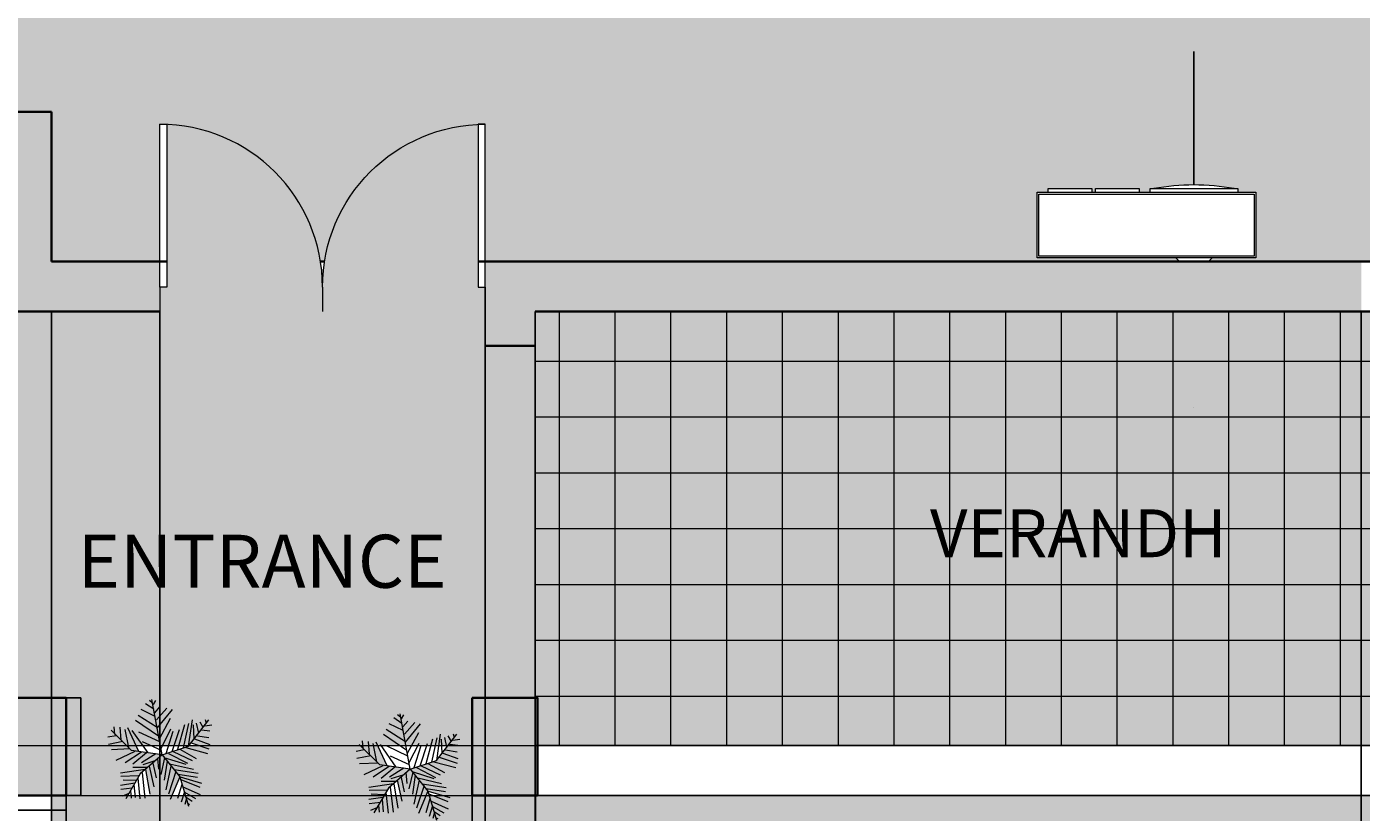
# Model space of a CAD drawing. Units: millimetres. Extents: x -229 to 16545, y -10488 to 4272.
# Tile 7 of 29: x 5862 to 12015, y -7746 to -4126. Entities that reach past the tile are written whole.
import ezdxf

# ---------------------------------------------------------------- set-up
doc = ezdxf.new("R2010")
doc.units = ezdxf.units.MM
for name, color, linetype, lineweight in [('A-ANNO-DIMS', 2, 'Continuous', 18), ('A-AREA-IDEN', 7, 'Continuous', 18), ('A-COLS', 7, 'Continuous', 35), ('A-DOOR', 4, 'Continuous', 18), ('A-FLOR-STRS', 7, 'Continuous', 18), ('A-FURN', 8, 'Continuous', 18), ('A-WALL', 7, 'Continuous', 35), ('L-PLNT-BEDS', 82, 'Continuous', 18), ('L-PLNT-TREE', 80, 'Continuous', 18), ('L-PVMT', 7, 'Continuous', 18), ('L-PVMT-JNTS', 8, 'Continuous', 13)]:
    doc.layers.add(name, color=color, linetype=linetype, lineweight=lineweight)
for name, color, linetype, lineweight, true_color in [('A-FLOR-PATT', 254, 'Continuous', 13, 0xfeeab9), ('A-FLOR-STRS-PATT', 51, 'Continuous', 13, 0xf8f6b0), ('A-WALL-PATT', 18, 'Continuous', 13, 0x000000), ('L-PLNT-PATT', 116, 'Continuous', 13, 0x136734), ('L-PVMT-PATT', 252, 'Continuous', 13, 0x939598)]:
    doc.layers.add(name, color=color, linetype=linetype, lineweight=lineweight, true_color=true_color)
doc.styles.get("Standard").update_dxf_attribs({"font": 'arial.ttf'})
doc.dimstyles.get("Standard").update_dxf_attribs({"dimtxt": 0.18, "dimasz": 0.18, "dimexe": 0.18, "dimexo": 0.0625, "dimgap": 0.09, "dimtad": 0, "dimtih": 1, "dimtoh": 1, "dimdec": 4, "dimzin": 0, "dimdsep": 46, "dimtxsty": 'Standard', "dimcen": 0.09, "dimadec": 0, "dimazin": 0, "dimtfac": 1, "dimtdec": 4, "dimtofl": 0, "dimtmove": 0, "dimatfit": 3, "dimfxl": 1, "dimtolj": 1, "dimtzin": 0, "dimarcsym": 0})

# ---------------------------------------------------------------- blocks, each defined once
blk = doc.blocks.new('Entertainment Center')
for p, q in [((-4, 0), (-5, -1)), ((4, 0), (-4, 0)), ((5, -1), (4, 0)), ((-17, -19), (-17, -1)), ((-17, -1), (43, -1)), ((-16.5, -18.5), (-16.5, -1.5)), ((-16.5, -1.5), (42.5, -1.5)), ((42.5, -1.5), (42.5, -18.5)), ((43, -1), (43, -19)), ((43, -19), (-17, -19)), ((42.5, -18.5), (-16.5, -18.5)), ((-12, -20), (-12, -19)), ((12, -20), (-12, -20)), ((12, -19), (12, -20)), ((15, -20), (15, -19)), ((27, -20), (15, -20)), ((27, -19), (27, -20)), ((28, -20), (28, -19)), ((40, -20), (28, -20)), ((40, -19), (40, -20))]:
    blk.add_line(p, q)
blk.add_arc((0, 40), 61, 259.6111, 280.3889)
blk = doc.blocks.new('*U12')
for p, q in [((0, 0), (0, -6)), ((40, 0), (40, -6))]:
    blk.add_line(p, q)
blk.add_lwpolyline([(0, 0), (0, 40), (1.75, 40), (1.75, 0)], close=True)
blk.add_arc((0, 0), 40, 0, 90)
blk = doc.blocks.new('*U18')
for p, q in [((-10.186, 53.64), (-13.084, 55.962)), ((0, 0), (-10.5, 57)), ((-9.099, 51.782), (-6.563, 55.962)), ((-7.288, 39.707), (-21.778, 46.673)), ((-8.737, 47.138), (-17.069, 52.711)), ((-7.65, 43.423), (-2.578, 49.46)), ((-5.839, 35.992), (4.667, 48.067)), ((-5.114, 27.632), (10.463, 46.673)), ((-48.585, 21.131), (-49.309, 29.026)), ((-43.513, 28.561), (-42.427, 15.558)), ((-35.544, 28.097), (-24.314, 3.947)), ((-3.665, 19.273), (-27.574, 35.527)), ((-5.114, 28.097), (-24.676, 40.636)), ((-2.941, 16.486), (8.652, 37.85)), ((16.259, 5.805), (23.142, 31.348)), ((22.055, 7.198), (27.489, 32.277)), ((27, 9), (48, 36)), ((27.127, 9.056), (31.112, 35.992)), ((31.836, 30.883), (32.561, 16.486)), ((35.096, 32.741), (37.27, 22.524)), ((38.719, 34.134), (41.979, 28.561)), ((43.791, 29.954), (51.036, 30.883)), ((44.153, 36.456), (45.239, 32.741)), ((-47.498, 19.737), (-55.83, 18.344)), ((-31.5, 4.5), (-52.5, 25.5)), ((-38.442, 26.239), (-34.819, 7.663)), ((-14.533, 2.09), (-30.834, 25.31)), ((-24.314, 23.917), (-2.941, 13.7)), ((-1.129, 6.734), (9.014, 26.704)), ((3.942, 1.625), (11.187, 24.381)), ((10.101, 3.483), (17.708, 26.239)), ((33.285, 16.486), (48.862, 10.913)), ((36.183, 19.737), (48.137, 17.88)), ((40.53, 25.775), (48.862, 24.846)), ((-40.615, 13.7), (-55.105, 10.913)), ((-33.37, 6.269), (-52.207, 5.34)), ((-28.299, 3.483), (-47.86, -5.805)), ((-21.416, 3.018), (-38.079, -8.128)), ((0, 0), (-31.5, 4.5)), ((-15.982, 2.09), (-30.11, -9.521)), ((0, 0), (-22.5, -19.5)), ((-6.563, 1.161), (-21.416, -8.128)), ((-20.691, 13.7), (-1.129, 4.876)), ((0, 0), (27, 9)), ((0, 0), (18, -22.5)), ((6.478, 1.625), (26.04, -8.592)), ((11.187, 3.483), (30.749, -5.805)), ((18.07, 5.805), (35.096, -3.483)), ((24.229, 7.663), (46.688, 1.625)), ((29.662, 12.307), (48.137, 6.269)), ((-15.257, -12.772), (-30.11, -12.772)), ((-6.563, -5.805), (-19.967, -9.985)), ((-13.446, -11.378), (-8.737, -32.741)), ((-9.461, -8.592), (-6.201, -23.453)), ((-4.752, -3.483), (-3.665, -14.629)), ((2.493, -3.019), (-1.491, -20.202)), ((1.769, -2.555), (24.229, -9.521)), ((5.029, -6.27), (2.131, -25.775)), ((9.014, -11.378), (3.58, -35.992)), ((7.565, -9.056), (32.198, -14.629)), ((-17.431, -15.094), (-42.789, -18.809)), ((-24.314, -21.596), (-42.427, -22.06)), ((-26.849, -26.24), (-40.253, -25.775)), ((-22.5, -19.5), (-37.5, -45)), ((-25.038, -23.918), (-22.865, -45.281)), ((-20.691, -18.345), (-17.793, -44.352)), ((-17.069, -15.094), (-12.721, -40.172)), ((14.085, -16.951), (6.478, -40.172)), ((18.07, -22.524), (8.289, -45.745)), ((12.274, -15.094), (36.907, -18.809)), ((16.259, -19.738), (36.183, -22.989)), ((18, -22.5), (27, -52.5)), ((18.433, -22.524), (40.53, -29.026)), ((19.157, -25.311), (38.719, -33.206)), ((-28.299, -29.026), (-42.789, -31.348)), ((-30.834, -34.135), (-42.427, -35.528)), ((-34.457, -39.708), (-40.978, -42.494)), ((-32.646, -36.921), (-31.921, -44.352)), ((-29.023, -30.884), (-27.936, -43.887)), ((20.244, -30.419), (15.897, -44.816)), ((22.78, -37.85), (19.519, -48.532)), ((21.331, -32.741), (39.081, -40.636)), ((22.78, -38.314), (34.372, -44.816)), ((24.591, -45.745), (23.142, -50.854)), ((24.591, -43.423), (30.749, -47.603)), ((26.764, -49.925), (28.213, -50.854))]:
    blk.add_line(p, q)
blk = doc.blocks.new('COL-300x450')
at = {"transparency": 33554615}
h = blk.add_hatch(color=256, dxfattribs=at)
h.dxf.hatch_style = 1
h.paths.add_polyline_path([(300, 450), (0, 450), (0, 0), (300, 0)])
at = {"transparency": 33554687}
blk.add_lwpolyline([(0, 450), (300, 450), (300, 0), (0, 0)], close=True, dxfattribs=at)
blk = doc.blocks.new('*D23')
at = {"layer": 'A-ANNO-DIMS', "color": 0, "lineweight": -2, "transparency": 16777216}
for p, q in [((6043.9, -7218.3), (6111.5, -7218.3)), ((6111.4, -7218.5), (6111.4, -7443.1)), ((6111.4, -7668.1), (6111.4, -7443.5)), ((6043.9, -7668.3), (6111.5, -7668.3))]:
    blk.add_line(p, q, dxfattribs=at)
at = {"layer": 'A-ANNO-DIMS', "color": 0, "transparency": 16777216}
for points in [[(6111.3, -7218.5), (6111.4, -7218.5), (6111.4, -7218.3)], [(6111.3, -7668.1), (6111.4, -7668.1), (6111.4, -7668.3)]]:
    blk.add_solid(points, dxfattribs=at)
at = {"layer": 'Defpoints', "color": 0, "transparency": 16777216}
for p in [(6043.9, -7218.3), (6111.4, -7218.3), (6043.9, -7668.3)]:
    blk.add_point(p, dxfattribs=at)
at = {"layer": 'A-ANNO-DIMS', "color": 0, "transparency": 16777216, "insert": (6111.4, -7443.3), "char_height": 0.18, "attachment_point": 5}
blk.add_mtext('\\A1;COLUMN 450 TYP.', dxfattribs=at)
blk = doc.blocks.new('*D24')
at = {"layer": 'A-ANNO-DIMS', "color": 0, "lineweight": -2, "transparency": 16777216}
for p, q in [((5743.9, -7668.3), (5743.9, -7736)), ((6043.9, -7668.3), (6043.9, -7736)), ((5744, -7735.8), (5893.3, -7735.8)), ((6043.7, -7735.8), (5894.5, -7735.8))]:
    blk.add_line(p, q, dxfattribs=at)
at = {"layer": 'A-ANNO-DIMS', "color": 0, "transparency": 16777216}
for points in [[(5744, -7735.7), (5744, -7735.8), (5743.9, -7735.8)], [(6043.7, -7735.7), (6043.7, -7735.8), (6043.9, -7735.8)]]:
    blk.add_solid(points, dxfattribs=at)
at = {"layer": 'Defpoints', "color": 0, "transparency": 16777216}
for p in [(5743.9, -7668.3), (6043.9, -7668.3), (6043.9, -7735.8)]:
    blk.add_point(p, dxfattribs=at)
at = {"layer": 'A-ANNO-DIMS', "color": 0, "transparency": 16777216, "insert": (5893.9, -7735.8), "char_height": 0.18, "attachment_point": 5}
blk.add_mtext('\\A1;300 TYP.', dxfattribs=at)
blk = doc.blocks.new('*D60')
at = {"layer": 'A-ANNO-DIMS', "color": 0, "lineweight": -2, "transparency": 16777216}
for p, q in [((8205.9, -7438.3), (8205.9, -10230.2)), ((14015.9, -7438.3), (14015.9, -10230.2)), ((8206.1, -10230), (11110.6, -10230)), ((14015.8, -10230), (11111.3, -10230))]:
    blk.add_line(p, q, dxfattribs=at)
at = {"layer": 'A-ANNO-DIMS', "color": 0, "transparency": 16777216}
for points in [[(8206.1, -10230), (8206.1, -10230.1), (8205.9, -10230)], [(14015.8, -10230), (14015.8, -10230.1), (14015.9, -10230)]]:
    blk.add_solid(points, dxfattribs=at)
at = {"layer": 'Defpoints', "color": 0, "transparency": 16777216}
for p in [(8205.9, -7438.3), (14015.9, -7438.3), (14015.9, -10230)]:
    blk.add_point(p, dxfattribs=at)
at = {"layer": 'A-ANNO-DIMS', "color": 0, "transparency": 16777216, "insert": (11110.9, -10230), "char_height": 0.18, "attachment_point": 5}
blk.add_mtext('\\A1;5810', dxfattribs=at)
blk = doc.blocks.new('*D61')
at = {"layer": 'A-ANNO-DIMS', "color": 0, "lineweight": -2, "transparency": 16777216}
for p, q in [((8206, -5438.3), (16544.5, -5438.3)), ((16544.3, -5438.5), (16544.3, -6438.1)), ((16544.3, -7438.1), (16544.3, -6438.5)), ((8206, -7438.3), (16544.5, -7438.3))]:
    blk.add_line(p, q, dxfattribs=at)
at = {"layer": 'A-ANNO-DIMS', "color": 0, "transparency": 16777216}
for points in [[(16544.3, -5438.5), (16544.4, -5438.5), (16544.3, -5438.3)], [(16544.3, -7438.1), (16544.4, -7438.1), (16544.3, -7438.3)]]:
    blk.add_solid(points, dxfattribs=at)
at = {"layer": 'Defpoints', "color": 0, "transparency": 16777216}
for p in [(8205.9, -5438.3), (16544.3, -5438.3), (8205.9, -7438.3)]:
    blk.add_point(p, dxfattribs=at)
at = {"layer": 'A-ANNO-DIMS', "color": 0, "transparency": 16777216, "insert": (16544.3, -6438.3), "char_height": 0.18, "attachment_point": 5}
blk.add_mtext('\\A1;2000', dxfattribs=at)
blk = doc.blocks.new('*D63')
at = {"layer": 'A-ANNO-DIMS', "color": 0, "lineweight": -2, "transparency": 16777216}
for p, q in [((6475.9, -5438.3), (6475.9, -10230.2)), ((7975.9, -5438.3), (7975.9, -10230.2)), ((6476.1, -10230), (7225.6, -10230)), ((7975.8, -10230), (7226.3, -10230))]:
    blk.add_line(p, q, dxfattribs=at)
at = {"layer": 'A-ANNO-DIMS', "color": 0, "transparency": 16777216}
for points in [[(6476.1, -10230), (6476.1, -10230.1), (6475.9, -10230)], [(7975.8, -10230), (7975.8, -10230.1), (7975.9, -10230)]]:
    blk.add_solid(points, dxfattribs=at)
at = {"layer": 'Defpoints', "color": 0, "transparency": 16777216}
for p in [(6475.9, -5438.3), (7975.9, -5438.3), (7975.9, -10230)]:
    blk.add_point(p, dxfattribs=at)
at = {"layer": 'A-ANNO-DIMS', "color": 0, "transparency": 16777216, "insert": (7225.9, -10230), "char_height": 0.18, "attachment_point": 5}
blk.add_mtext('\\A1;1500', dxfattribs=at)
blk = doc.blocks.new('*D79')
at = {"layer": 'A-ANNO-DIMS', "color": 0, "lineweight": -2, "transparency": 16777216}
for p, q in [((8206, -7668.3), (16544.5, -7668.3)), ((16544.3, -7668.5), (16544.3, -8458.1)), ((16544.3, -9248.1), (16544.3, -8458.5)), ((8209.2, -9248.3), (16544.5, -9248.3))]:
    blk.add_line(p, q, dxfattribs=at)
at = {"layer": 'A-ANNO-DIMS', "color": 0, "transparency": 16777216}
for points in [[(16544.3, -7668.5), (16544.4, -7668.5), (16544.3, -7668.3)], [(16544.3, -9248.1), (16544.4, -9248.1), (16544.3, -9248.3)]]:
    blk.add_solid(points, dxfattribs=at)
at = {"layer": 'Defpoints', "color": 0, "transparency": 16777216}
for p in [(8205.9, -7668.3), (8209.2, -9248.3), (16544.3, -9248.3)]:
    blk.add_point(p, dxfattribs=at)
at = {"layer": 'A-ANNO-DIMS', "color": 0, "transparency": 16777216, "insert": (16544.3, -8458.3), "char_height": 0.18, "attachment_point": 5}
blk.add_mtext('\\A1;1580', dxfattribs=at)
blk = doc.blocks.new('*D80')
at = {"layer": 'A-ANNO-DIMS', "color": 0, "lineweight": -2, "transparency": 16777216}
for p, q in [((6043.9, -7218.3), (6043.9, -10230.2)), ((7916.5, -7218.3), (7916.5, -10230.2)), ((6044, -10230), (6979.7, -10230)), ((7916.3, -10230), (6980.6, -10230))]:
    blk.add_line(p, q, dxfattribs=at)
at = {"layer": 'A-ANNO-DIMS', "color": 0, "transparency": 16777216}
for points in [[(6044, -10230), (6044, -10230.1), (6043.9, -10230)], [(7916.3, -10230), (7916.3, -10230.1), (7916.5, -10230)]]:
    blk.add_solid(points, dxfattribs=at)
at = {"layer": 'Defpoints', "color": 0, "transparency": 16777216}
for p in [(6043.9, -7218.3), (7916.5, -7218.3), (7916.5, -10230)]:
    blk.add_point(p, dxfattribs=at)
at = {"layer": 'A-ANNO-DIMS', "color": 0, "transparency": 16777216, "insert": (6980.2, -10230), "char_height": 0.18, "attachment_point": 5}
blk.add_mtext('\\A1;1872.6', dxfattribs=at)
blk = doc.blocks.new('*D86')
at = {"layer": 'A-ANNO-DIMS', "color": 0, "lineweight": -2, "transparency": 16777216}
for p, q in [((8205.9, -5438.3), (8205.9, -10230.2)), ((12015.2, -5438.3), (12015.2, -10230.2)), ((8206.1, -10230), (10110.2, -10230)), ((12015, -10230), (10110.9, -10230))]:
    blk.add_line(p, q, dxfattribs=at)
at = {"layer": 'A-ANNO-DIMS', "color": 0, "transparency": 16777216}
for points in [[(8206.1, -10230), (8206.1, -10230.1), (8205.9, -10230)], [(12015, -10230), (12015, -10230.1), (12015.2, -10230)]]:
    blk.add_solid(points, dxfattribs=at)
at = {"layer": 'Defpoints', "color": 0, "transparency": 16777216}
for p in [(8205.9, -5438.3), (12015.2, -5438.3), (8205.9, -10230)]:
    blk.add_point(p, dxfattribs=at)
at = {"layer": 'A-ANNO-DIMS', "color": 0, "transparency": 16777216, "insert": (10110.6, -10230), "char_height": 0.18, "attachment_point": 5}
blk.add_mtext('\\A1;3809', dxfattribs=at)
blk = doc.blocks.new('*D90')
at = {"layer": 'A-ANNO-DIMS', "color": 0, "lineweight": -2, "transparency": 16777216}
for p, q in [((5975.9, -5438.3), (5975.9, -10230.2)), ((6475.9, -5438.3), (6475.9, -10230.2)), ((5976.1, -10230), (6225.6, -10230)), ((6475.8, -10230), (6226.2, -10230))]:
    blk.add_line(p, q, dxfattribs=at)
at = {"layer": 'A-ANNO-DIMS', "color": 0, "transparency": 16777216}
for points in [[(5976.1, -10230), (5976.1, -10230.1), (5975.9, -10230)], [(6475.8, -10230), (6475.8, -10230.1), (6475.9, -10230)]]:
    blk.add_solid(points, dxfattribs=at)
at = {"layer": 'Defpoints', "color": 0, "transparency": 16777216}
for p in [(5975.9, -5438.3), (6475.9, -5438.3), (6475.9, -10230)]:
    blk.add_point(p, dxfattribs=at)
at = {"layer": 'A-ANNO-DIMS', "color": 0, "transparency": 16777216, "insert": (6225.9, -10230), "char_height": 0.18, "attachment_point": 5}
blk.add_mtext('\\A1;500', dxfattribs=at)
blk = doc.blocks.new('*D105')
at = {"layer": 'A-ANNO-DIMS', "color": 0, "lineweight": -2, "transparency": 16777216}
for p, q in [((11243.7, -4240.2), (11243.5, -4240.2)), ((11243.5, -4240.2), (11243.5, -4855.1)), ((11243.4, -5880.6), (11243.6, -5880.6)), ((11243.5, -5880.6), (11243.5, -5880.5))]:
    blk.add_line(p, q, dxfattribs=at)
at = {"layer": 'A-ANNO-DIMS', "color": 0, "transparency": 16777216}
blk.add_solid([(11243.4, -4855.1), (11243.5, -4855.1), (11243.5, -4855.3)], dxfattribs=at)
at = {"layer": 'Defpoints', "color": 0, "transparency": 16777216}
for p in [(11243.5, -4855.3), (11243.5, -5880.6)]:
    blk.add_point(p, dxfattribs=at)
at = {"layer": 'A-ANNO-DIMS', "color": 0, "transparency": 16777216, "insert": (11244.4, -4240.2), "char_height": 0.18, "attachment_point": 5}
blk.add_mtext('\\A1;2X R1025.2', dxfattribs=at)

msp = doc.modelspace()

# ---------------------------------------------------------------- hatches: boundary and pattern name
at = {"layer": 'A-FLOR-PATT', "transparency": 33554592}
h = msp.add_hatch(color=256, dxfattribs=at)
h.dxf.hatch_style = 1
h.paths.add_polyline_path([(7975.933, -5325.772), (7943.121, -5325.772), (7943.121, -4576.49, 0.40145271), (7225.933, -5325.772, 0.40145271), (6508.746, -4576.49), (6508.746, -5325.772), (6475.933, -5325.772), (6475.933, -5438.272), (5975.933, -5438.272), (5975.933, -7267.724), (5975.933, -7438.272), (6478.619, -7438.272), (6463.448, -7355.919), (6464.88, -7356.837), (6463.849, -7358.097), (6478.619, -7438.272), (6610.327, -7438.272), (6632.656, -7409.564), (6632.525, -7406.967), (6634.208, -7407.569), (6619.273, -7426.77), (6654.466, -7438.272), (7610.517, -7438.272), (7607.41, -7421.409), (7608.842, -7422.327), (7607.812, -7423.587), (7610.517, -7438.272), (7975.933, -7438.272)])
h.paths.add_polyline_path([(13785.933, -1208.272), (9555.933, -1208.272), (9555.933, -961.785), (9705.933, -961.785), (9705.933, -918.035), (10704.976, -918.035, 0.40145271), (9705.933, 38.215), (9555.933, 38.215), (9555.933, 2021.728), (5975.933, 2021.728), (5975.933, 755.492), (5745.933, 755.492), (5745.933, 1427.266), (2918.813, 1427.266), (2918.813, -492.942), (5013.319, -492.942), (5013.319, -978.272), (5745.933, -978.272), (5745.933, -397.513), (5975.933, -397.513), (5975.933, -1208.272), (4560.933, -1208.272), (4560.933, -1265.772), (4448.433, -1265.772), (4448.433, -1298.585), (4445.933, -1298.585), (3699.151, -1298.585, 0.40145271), (4448.433, -2015.772), (4560.933, -2015.772), (4560.933, -2384.177), (5745.933, -2384.177), (5799.402, -2384.177), (5799.402, -4518.272), (5975.933, -4518.272), (5975.933, -5208.272), (6475.933, -5208.272), (6475.933, -4575.772), (6508.746, -4575.772), (6508.746, -4576.49, -0.35647263), (7216.672, -5208.272), (7235.194, -5208.272, -0.35647263), (7943.121, -4576.49), (7943.121, -4575.772), (7975.933, -4575.772), (7975.933, -5208.272), (11176.247, -5208.272), (11159.44, -5191.465), (10520.768, -5191.465), (10520.768, -4888.936), (10571.19, -4888.936), (10571.19, -4872.129), (10772.876, -4872.129), (10772.876, -4888.936), (10789.683, -4888.936), (10789.683, -4872.129), (10991.368, -4872.129), (10991.368, -4888.936), (11041.79, -4888.936), (11041.79, -4872.129), (11058.597, -4872.129, -0.09090909), (11428.354, -4872.129), (11445.162, -4872.129), (11445.162, -4888.936), (11529.197, -4888.936), (11529.197, -5191.465), (11327.512, -5191.465), (11310.704, -5208.272), (13785.933, -5208.272)])
h.paths.add_polyline_path([(11047.216, -1630.944, -1), (11402.816, -1630.944, -1)], flags=16)
h.paths.add_polyline_path([(11148.816, -1630.944), (11225.016, -1554.744), (11301.216, -1630.944), (11225.016, -1707.144)], flags=0)
h.paths.add_polyline_path([(11199.616, -1630.944, -1), (11250.416, -1630.944, -1)], flags=0)
h.paths.add_polyline_path([(11588.751, -2096.259), (11588.751, -1543.254, -0.26666697), (12864.918, -1543.254), (12864.918, -2096.259), (12737.302, -2096.259), (12737.302, -2063.121), (11716.368, -2063.121), (11716.368, -2096.259)], flags=16)
h.paths.add_polyline_path([(12012.696, -2489.42), (12600.997, -2489.42), (12600.997, -3666.022), (12012.696, -3666.022)], flags=16)
h.paths.add_polyline_path([(12176.41, -3599.403), (12174.938, -3609.076), (12173.789, -3618.819), (12173.09, -3628.559), (12172.973, -3638.221), (12173.89, -3652.852), (12175.008, -3657.025), (12172.909, -3643.473), (12173.142, -3624.297), (12175.386, -3605.273)], flags=0)
h.paths.add_polyline_path([(8026.289, -286.944), (7737.703, -287.19), (7734.87, -269.156), (8029.092, -268.905)], flags=16)
h.paths.add_polyline_path([(7733.453, -260.139), (7710.784, -115.865), (7557.191, -115.996), (7556.999, 109.744), (7412.687, 132.166), (7412.433, 429.206), (7556.707, 451.876), (7556.568, 614.769), (7412.256, 637.19), (7412.003, 934.231), (7556.276, 956.9), (7556.084, 1182.639), (7709.677, 1182.77), (7732.099, 1327.082), (8029.14, 1327.335), (8051.808, 1183.062), (8205.401, 1183.192), (8205.594, 957.454), (8349.906, 935.031), (8350.159, 637.99), (8205.885, 615.322), (8206.024, 452.43), (8350.336, 430.006), (8350.59, 132.965), (8206.316, 110.298), (8206.509, -115.442), (8052.916, -115.573), (8030.493, -259.885)], flags=16)
h.paths.add_polyline_path([(12261.416, -3475.554), (12262.632, -3486.776), (12264.032, -3497.007), (12265.554, -3506.365), (12267.136, -3514.968), (12268.719, -3522.935), (12271.304, -3535.59), (12273.606, -3548.078), (12275.271, -3561.064), (12275.93, -3574.938), (12275.325, -3590.3), (12273.425, -3607.964), (12270.795, -3625.658), (12268.066, -3641.063), (12266.318, -3649.679), (12265.456, -3653.626), (12263.984, -3659.846), (12264.032, -3659.566), (12264.342, -3658.241), (12264.807, -3656.37), (12265.456, -3653.626), (12266.318, -3649.679), (12267.409, -3644.302), (12268.668, -3637.664), (12270.019, -3630.037), (12271.384, -3621.695), (12272.69, -3612.908), (12273.857, -3603.948), (12274.81, -3595.088), (12275.47, -3586.601), (12275.782, -3578.689), (12275.757, -3571.292), (12275.423, -3564.275), (12274.816, -3557.512), (12273.964, -3550.872), (12272.896, -3544.224), (12271.645, -3537.439), (12270.24, -3530.385), (12267.543, -3517.181), (12264.612, -3501.247), (12261.849, -3481.059)], flags=0)
h.paths.add_polyline_path([(12332.136, -3408.03), (12333.483, -3416.79), (12335.077, -3424.54), (12336.915, -3431.355), (12338.991, -3437.32), (12341.266, -3442.55), (12343.694, -3447.166), (12346.229, -3451.292), (12348.826, -3455.051), (12351.438, -3458.563), (12357.476, -3466.491), (12363.61, -3476.575), (12368.309, -3489.762), (12369.929, -3503.427), (12369.842, -3516.511), (12368.43, -3530.867), (12365.816, -3545.835), (12362.382, -3559.786), (12360.968, -3564.487), (12363.063, -3557.021), (12364.898, -3549.566), (12366.473, -3542.077), (12367.773, -3534.631), (12368.781, -3527.301), (12369.483, -3520.162), (12369.863, -3513.291), (12369.906, -3506.759), (12369.599, -3500.643), (12368.93, -3494.999), (12367.924, -3489.796), (12366.61, -3484.994), (12365.024, -3480.542), (12363.19, -3476.399), (12361.141, -3472.516), (12358.909, -3468.847), (12356.525, -3465.347), (12354.02, -3461.954), (12351.438, -3458.563), (12345.462, -3450.529), (12339.923, -3439.996), (12335.85, -3428.296), (12332.68, -3412.888)], flags=0)
h.paths.add_polyline_path([(12385.287, -3334.612), (12384.977, -3342.409), (12385.02, -3349.196), (12385.4, -3355.066), (12386.104, -3360.105), (12387.112, -3364.41), (12388.412, -3368.071), (12389.987, -3371.181), (12391.823, -3373.832), (12393.919, -3376.097), (12396.337, -3377.978), (12399.153, -3379.462), (12402.445, -3380.531), (12406.289, -3381.172), (12410.758, -3381.371), (12415.935, -3381.106), (12421.893, -3380.368), (12428.658, -3379.159), (12436.069, -3377.55), (12443.907, -3375.635), (12451.961, -3373.505), (12460.015, -3371.254), (12467.853, -3368.971), (12475.263, -3366.749), (12482.029, -3364.68), (12491.877, -3361.657), (12497.701, -3360.107), (12501.639, -3359.288), (12510.135, -3358.326), (12519.662, -3365.412), (12524.243, -3378.911), (12523.764, -3390.7), (12520.746, -3401.577), (12514.248, -3415.634), (12511.518, -3420.418), (12515.856, -3412.154), (12519.153, -3405.024), (12521.516, -3398.804), (12523.049, -3393.276), (12523.865, -3388.212), (12524.059, -3383.441), (12523.7, -3378.958), (12522.853, -3374.815), (12521.576, -3371.054), (12519.931, -3367.722), (12517.982, -3364.865), (12515.786, -3362.529), (12513.405, -3360.758), (12510.877, -3359.588), (12508.136, -3358.982), (12505.086, -3358.897), (12501.639, -3359.288), (12497.701, -3360.107), (12493.183, -3361.309), (12487.988, -3362.851), (12476.403, -3366.408), (12463.335, -3370.326), (12447.372, -3374.788), (12431.759, -3378.604), (12418.504, -3380.974), (12405.811, -3381.624), (12394.725, -3378.025), (12388.039, -3368.367), (12385.583, -3357.877), (12384.826, -3346.204), (12385.428, -3331.059), (12385.953, -3325.719)], flags=0)
h.paths.add_polyline_path([(7880.016, 1173.969), (7880.373, 1175.495), (7880.433, 1175.851), (7879.484, 1171.818)], flags=0)
h.paths.add_polyline_path([(7802.33, 874.962), (7800.771, 885.032), (7798.932, 893.941), (7796.811, 901.774), (7794.419, 908.63), (7791.798, 914.639), (7789.002, 919.945), (7786.083, 924.686), (7783.093, 929.005), (7780.087, 933.043), (7774.996, 939.717), (7768.406, 949.37), (7762.174, 963.427), (7759.342, 978.002), (7758.629, 991.888), (7759.492, 1007.928), (7761.801, 1025.496), (7765.392, 1044.035), (7766.625, 1049.048), (7764.522, 1039.543), (7762.719, 1030.232), (7761.232, 1021.168), (7760.08, 1012.405), (7759.28, 1003.994), (7758.849, 995.988), (7758.806, 988.44), (7759.167, 981.404), (7759.942, 974.914), (7761.104, 968.936), (7762.617, 963.414), (7764.448, 958.299), (7766.559, 953.535), (7768.918, 949.073), (7771.487, 944.856), (7774.232, 940.835), (7777.115, 936.938), (7782.377, 930.041), (7787.845, 922.139), (7793.348, 911.698), (7798.042, 898.247), (7801.702, 880.527)], flags=0)
h.paths.add_polyline_path([(12519.068, -3228.534), (12519.615, -3236.235), (12520.529, -3242.343), (12521.78, -3247.103), (12523.337, -3250.758), (12525.171, -3253.556), (12527.248, -3255.709), (12529.522, -3257.296), (12531.95, -3258.361), (12534.486, -3258.949), (12537.082, -3259.11), (12539.694, -3258.888), (12542.277, -3258.329), (12544.781, -3257.478), (12547.173, -3256.388), (12549.46, -3255.129), (12550.455, -3254.517), (12555.825, -3251.109), (12557.835, -3249.942), (12565.181, -3246.404), (12574.565, -3253.032), (12576.931, -3265.022), (12576.627, -3277.425), (12575.416, -3290.819), (12574.851, -3295.392), (12575.708, -3287.593), (12576.322, -3280.806), (12576.688, -3274.939), (12576.812, -3269.899), (12576.688, -3265.593), (12576.322, -3261.932), (12575.708, -3258.822), (12574.851, -3256.172), (12573.753, -3253.905), (12572.439, -3252.005), (12570.943, -3250.474), (12569.293, -3249.309), (12567.523, -3248.513), (12565.658, -3248.083), (12563.732, -3248.022), (12561.777, -3248.328), (12559.814, -3248.989), (12557.835, -3249.942), (12555.825, -3251.109), (12553.77, -3252.413), (12551.652, -3253.78), (12549.46, -3255.129), (12543.167, -3258.594), (12532.661, -3259.485), (12524.685, -3253.923), (12520.949, -3245.152), (12519.138, -3233.042)], flags=0)
h.paths.add_polyline_path([(7741.293, 790.501), (7741.641, 799.467), (7741.584, 807.269), (7741.141, 814.015), (7740.329, 819.809), (7739.165, 824.757), (7737.667, 828.966), (7735.853, 832.541), (7733.74, 835.586), (7731.348, 838.188), (7728.71, 840.348), (7725.861, 842.052), (7722.836, 843.28), (7719.671, 844.015), (7716.4, 844.237), (7713.06, 843.932), (7709.684, 843.081), (7706.304, 841.686), (7702.923, 839.834), (7699.543, 837.629), (7696.164, 835.178), (7692.784, 832.585), (7684.718, 826.315), (7675.609, 820.63), (7664.001, 817.274), (7654.105, 821.884), (7647.171, 832.02), (7644.191, 846.522), (7646.321, 860.288), (7647.49, 864.223), (7645.946, 857.865), (7645.046, 852.044), (7644.827, 846.557), (7645.243, 841.404), (7646.221, 836.642), (7647.693, 832.318), (7649.587, 828.489), (7651.832, 825.206), (7654.359, 822.523), (7657.097, 820.49), (7659.984, 819.145), (7662.993, 818.452), (7666.108, 818.357), (7669.311, 818.809), (7672.583, 819.755), (7675.908, 821.139), (7679.268, 822.913), (7682.645, 825.021), (7686.025, 827.401), (7689.404, 829.958), (7692.784, 832.585), (7700.505, 838.509), (7709.871, 843.64), (7721.436, 844.698), (7733.277, 837.617), (7739.571, 825.214), (7741.557, 811.049), (7741.669, 795.575)], flags=0)
h.paths.add_polyline_path([(8377.641, 137.216), (8359.607, 134.382), (8359.356, 428.605), (8377.395, 425.802)], flags=16)
h.paths.add_polyline_path([(7650.715, 668.465), (7650.08, 677.319), (7649.023, 684.34), (7647.579, 689.811), (7645.785, 694.012), (7643.675, 697.228), (7641.286, 699.7), (7638.669, 701.521), (7635.876, 702.744), (7632.96, 703.419), (7629.974, 703.601), (7626.971, 703.344), (7624.004, 702.697), (7621.125, 701.717), (7618.375, 700.462), (7615.749, 699.013), (7614.561, 698.279), (7608.435, 694.382), (7606.125, 693.04), (7598.981, 689.594), (7589.669, 693.773), (7585.26, 702.856), (7584.221, 713.11), (7584.49, 724.584), (7585.863, 739.937), (7586.518, 745.277), (7585.539, 736.31), (7584.841, 728.507), (7584.424, 721.761), (7584.288, 715.966), (7584.433, 711.016), (7584.86, 706.807), (7585.567, 703.231), (7586.556, 700.186), (7587.821, 697.58), (7589.332, 695.397), (7591.053, 693.637), (7592.951, 692.3), (7594.989, 691.385), (7597.132, 690.895), (7599.346, 690.826), (7601.594, 691.18), (7603.851, 691.943), (7606.125, 693.04), (7608.435, 694.382), (7610.797, 695.885), (7613.229, 697.458), (7620.475, 701.929), (7632.001, 704.44), (7643.476, 699.417), (7648.536, 687.571), (7650.63, 673.661)], flags=0)
h.paths.add_polyline_path([(7385.628, 136.37), (7385.382, 424.956), (7403.416, 427.789), (7403.667, 133.567)], flags=16)
h.paths.add_polyline_path([(12993.884, -2257.186), (12959.588, -2257.186), (12959.588, -2125.099), (13531.966, -2125.099, -0.19047621), (13531.966, -3974.321), (12959.588, -3974.321), (12959.588, -3842.233), (12993.884, -3842.233)], flags=16)
h.paths.add_polyline_path([(13413.486, -3313.884), (13413.486, -2785.535), (13562.885, -2785.535, -0.04962821), (13562.885, -3313.884)], flags=0)
h.paths.add_polyline_path([(8377.21, 642.241), (8359.176, 639.407), (8358.925, 933.629), (8376.964, 930.826)], flags=16)
h.paths.add_polyline_path([(13086.058, -1864.83), (13086.058, -1449.84), (13501.048, -1449.84), (13501.048, -1864.83)], flags=16)
h.paths.add_polyline_path([(13305.814, -1862.197), (13302.103, -1859.624), (13298.088, -1857.068), (13293.799, -1854.536), (13289.262, -1852.031), (13284.504, -1849.559), (13279.554, -1847.125), (13274.439, -1844.735), (13269.17, -1842.389), (13263.701, -1840.081), (13257.97, -1837.797), (13251.914, -1835.525), (13245.472, -1833.252), (13238.582, -1830.968), (13231.18, -1828.66), (13223.206, -1826.315), (13209.182, -1822.458), (13204.584, -1821.48), (13217.962, -1824.773), (13235.072, -1829.804), (13248.777, -1834.349), (13260.829, -1838.869), (13274.479, -1844.63), (13289.675, -1852.101), (13302.553, -1859.704)], flags=0)
h.paths.add_polyline_path([(13428.104, -1820.994), (13419.007, -1818.141), (13409.95, -1815.4), (13400.766, -1812.747), (13391.271, -1810.151), (13376.087, -1806.251), (13370.618, -1805.019), (13386.304, -1808.794), (13405.087, -1813.928), (13423.014, -1819.354)], flags=0)
h.paths.add_polyline_path([(7385.197, 641.395), (7384.951, 929.98), (7402.986, 932.814), (7403.236, 638.592)], flags=16)
h.paths.add_polyline_path([(13262.537, -1725.526), (13253.246, -1724.74), (13244.516, -1724.117), (13235.94, -1723.625), (13223.267, -1723.062), (13217.598, -1722.912), (13231.966, -1723.397), (13248.733, -1724.359), (13266.899, -1725.895), (13272.802, -1726.502)], flags=0)
h.paths.add_polyline_path([(13191.893, -1641.137), (13208.675, -1640.506), (13214.057, -1640.258), (13197.763, -1640.936)], flags=0)
h.paths.add_polyline_path([(13097.524, -1608.457), (13114.284, -1609.031), (13120.126, -1609.105), (13103.045, -1608.71)], flags=0)
h.paths.add_polyline_path([(13465.328, -1521.577), (13473.906, -1517.015), (13481.761, -1511.636), (13492.562, -1502.076), (13495.327, -1497.933), (13485.818, -1508.858), (13470.208, -1519.547)], flags=0)
h.paths.add_polyline_path([(13175.015, -1500.891), (13184.046, -1501.807), (13192.721, -1502.52), (13201.114, -1503.034), (13209.273, -1503.351), (13217.244, -1503.476), (13225.078, -1503.41), (13232.821, -1503.16), (13240.524, -1502.728), (13248.233, -1502.117), (13255.993, -1501.322), (13263.825, -1500.293), (13271.746, -1498.974), (13279.775, -1497.305), (13287.928, -1495.229), (13296.222, -1492.688), (13304.675, -1489.622), (13313.304, -1485.975), (13322.089, -1481.727), (13330.859, -1477.028), (13339.408, -1472.063), (13347.526, -1467.02), (13355.006, -1462.087), (13364.86, -1455.202), (13367.224, -1453.299), (13358.544, -1459.754), (13343.348, -1469.775), (13326.143, -1479.767), (13309.023, -1488.045), (13292.249, -1494.129), (13276.009, -1498.264), (13260.299, -1500.88), (13244.401, -1502.51), (13228.945, -1503.378), (13213.316, -1503.508), (13197.047, -1502.876), (13180.088, -1501.481)], flags=0)
h.paths.add_polyline_path([(7733.501, 1336.101), (7736.303, 1354.14), (8024.889, 1354.386), (8027.723, 1336.352)], flags=16)
at = {"layer": 'A-FLOR-PATT', "transparency": 33554615}
h = msp.add_hatch(color=256, dxfattribs=at)
h.dxf.hatch_style = 1
h.paths.add_polyline_path([(5975.933, -5438.272), (5745.933, -5438.272), (5745.933, -7267.724), (5745.933, -7438.272), (5975.933, -7438.272)])
h = msp.add_hatch(color=256, dxfattribs=at)
h.dxf.hatch_style = 1
h.paths.add_polyline_path([(8205.933, -5596.884), (7975.933, -5596.884), (7975.933, -7438.272), (8205.933, -7438.272)])
at = {"layer": 'A-FLOR-STRS-PATT', "transparency": 33554615}
h = msp.add_hatch(color=256, dxfattribs=at)
h.dxf.hatch_style = 1
h.paths.add_polyline_path([(8209.16, -7668.272), (5975.933, -7668.272), (5975.933, -8003.395), (6096.954, -8003.395), (6116.245, -7994.236), (6180.362, -8003.395), (6237.45, -8003.395), (6215.763, -7885.666), (6217.195, -7886.584), (6216.164, -7887.844), (6237.45, -8003.395), (6264.12, -8003.395), (6359.981, -7971.442), (6384.971, -7939.312), (6384.84, -7936.715), (6386.523, -7937.317), (6360.638, -7970.597), (6360.54, -7971.255), (6344.488, -7976.606), (6444.134, -8003.395), (7862.582, -8003.395), (7881.873, -7994.236), (7945.991, -8003.395), (8003.078, -8003.395), (7981.391, -7885.666), (7982.823, -7886.584), (7981.793, -7887.844), (8003.078, -8003.395), (8029.748, -8003.395), (8125.609, -7971.442), (8150.599, -7939.312), (8150.468, -7936.715), (8152.151, -7937.317), (8209.16, -7864.019)])
h.paths.add_polyline_path([(6610.327, -7438.272), (6608.323, -7440.849), (6608.225, -7441.508), (6486.678, -7482.023), (6409.988, -7548.488), (6430.756, -7668.272), (6531.713, -7668.272), (6567.486, -7583.344), (6567.184, -7582.338), (6567.83, -7582.528), (6567.486, -7583.344), (6588.563, -7653.601), (6614.718, -7668.272), (7510.183, -7668.272), (7529.817, -7634.894), (7630.64, -7547.514), (7522.745, -7532.1), (7479.114, -7438.272)])
h.paths.add_polyline_path([(8205.933, -7438.272), (7805.227, -7438.272), (7752.285, -7506.34), (7752.188, -7506.998), (7630.64, -7547.514), (7570.616, -7599.535), (7585.768, -7668.272), (7703.261, -7668.272), (7711.448, -7648.835), (7711.146, -7647.829), (7780.622, -7668.272), (8205.933, -7668.272)])
h.paths.add_polyline_path([(6486.678, -7482.023), (6378.783, -7466.61), (6365.606, -7438.272), (5975.933, -7438.272), (5975.933, -7668.272), (6312.811, -7668.272), (6332.694, -7659.777), (6385.855, -7569.403)])
h.paths.add_polyline_path([(8004.621, -8011.771), (7945.991, -8003.395), (6264.12, -8003.395), (6238.993, -8011.771), (6162.303, -8078.236), (6162.466, -8079.176), (6160.964, -8079.396), (6238.993, -8011.771), (6180.362, -8003.395), (5975.933, -8003.395), (5975.933, -8317.848), (8209.16, -8317.848), (8209.16, -8003.395), (8029.748, -8003.395), (8004.621, -8011.771), (7927.931, -8078.236), (7928.094, -8079.176), (7926.592, -8079.396)])
h.paths.add_polyline_path([(6340.675, -8182.674), (6340.529, -8183.153), (6340.878, -8183.349)], flags=16)
h.paths.add_polyline_path([(8106.304, -8182.674), (8106.157, -8183.153), (8106.506, -8183.349)], flags=16)
h.paths.add_polyline_path([(7981.391, -8506.197), (7982.823, -8507.115), (7981.793, -8508.375), (8004.621, -8632.301), (8125.609, -8591.972), (8150.599, -8559.842), (8150.468, -8557.245), (8152.151, -8557.847), (8209.16, -8484.549), (8209.16, -8317.848), (5975.933, -8317.848), (5975.933, -8632.301), (6126.407, -8632.301), (6145.698, -8623.142), (6209.815, -8632.301), (6266.903, -8632.301), (6245.216, -8514.572), (6246.648, -8515.49), (6245.617, -8516.75), (6266.903, -8632.301), (6293.573, -8632.301), (6389.434, -8600.348), (6414.424, -8568.218), (6414.293, -8565.621), (6415.975, -8566.223), (6390.091, -8599.503), (6389.993, -8600.161), (6373.941, -8605.512), (6473.587, -8632.301), (7844.942, -8632.301), (7881.873, -8614.766), (8004.621, -8632.301)])
h.paths.add_polyline_path([(8004.621, -8632.301), (6293.573, -8632.301), (6268.446, -8640.677), (6191.756, -8707.142), (6191.919, -8708.082), (6190.417, -8708.302), (6268.446, -8640.677), (6209.815, -8632.301), (5975.933, -8632.301), (5975.933, -8946.754), (8209.16, -8946.754), (8209.16, -8632.301), (8004.621, -8632.301), (7927.931, -8698.766), (7928.094, -8699.706), (7926.592, -8699.926)])
h.paths.add_polyline_path([(6370.128, -8811.58), (6369.982, -8812.059), (6370.331, -8812.255)], flags=16)
h.paths.add_polyline_path([(8106.304, -8803.204), (8106.157, -8803.684), (8106.506, -8803.879)], flags=16)
h.paths.add_polyline_path([(8209.16, -8946.754), (5975.933, -8946.754), (5975.933, -9248.272), (8209.16, -9248.272)])
at = {"layer": 'A-WALL-PATT'}
h = msp.add_hatch(color=256, dxfattribs=at)
h.dxf.hatch_style = 1
h.paths.add_polyline_path([(7294.425, 2163.983), (7294.425, 2251.728), (4412.722, 2251.728), (4412.722, 2166.741), (4412.722, 2122.457), (4412.722, 2021.728), (7294.425, 2021.728), (7294.425, 2119.698)])
h.paths.add_polyline_path([(11407.51, 2166.741), (11407.51, 2251.728), (8296.763, 2251.728), (8296.763, 2163.983), (8296.763, 2119.698), (8296.763, 2021.728), (11407.51, 2021.728), (11407.51, 2122.457)])
h.paths.add_polyline_path([(9785.933, 2021.728), (9555.933, 2021.728), (9555.933, 38.215), (9705.933, 38.215, -0.02002407), (9785.933, 35.01)])
h.paths.add_polyline_path([(14015.933, 2251.728), (12488.002, 2251.728), (12488.002, 2166.742), (12488.002, 2122.738), (12488.002, 2021.728), (13785.933, 2021.728), (13785.933, -2305.465), (13883.903, -2305.465), (13928.188, -2305.465), (14015.933, -2305.465)])
h.paths.add_polyline_path([(13785.933, -978.272), (9785.933, -978.272), (9785.933, -961.785), (9705.933, -961.785), (9555.933, -961.785), (9555.933, -1208.272), (13785.933, -1208.272)])
h.paths.add_polyline_path([(5975.933, 2021.728), (5745.933, 2021.728), (5745.933, 755.492), (5975.933, 755.492)])
h.paths.add_polyline_path([(2245.933, 2021.728), (3420.865, 2021.728), (3420.865, 2122.457), (3420.865, 2167.104), (3420.865, 2251.728), (2015.933, 2251.728), (2015.933, -3326.811), (2100.943, -3326.811), (2155.199, -3326.811), (2245.933, -3326.811)])
h.paths.add_polyline_path([(5975.933, -397.513), (5745.933, -397.513), (5745.933, -978.272), (2245.933, -978.272), (2245.933, -1208.272), (5975.933, -1208.272)])
h.paths.add_polyline_path([(12015.17, -5208.272), (7975.933, -5208.272), (7975.933, -5325.772), (7975.933, -5438.272), (7975.933, -5596.884), (8205.933, -5596.884), (8205.933, -5438.272), (12015.17, -5438.272), (12015.17, -5337.543), (12015.17, -5293.259)])
h.paths.add_polyline_path([(5975.933, -4518.272), (4567.83, -4518.272), (4567.83, -4603.259), (4567.83, -4647.543), (4567.83, -4748.272), (5745.933, -4748.272), (5745.933, -5438.272), (5975.933, -5438.272), (6475.933, -5438.272), (6475.933, -5325.772), (6475.933, -5208.272), (5975.933, -5208.272)])
h.paths.add_polyline_path([(3765.491, -4518.272), (2245.933, -4518.272), (2245.933, -4748.272), (3765.491, -4748.272), (3765.491, -4647.543), (3765.491, -4603.259)])
at = {"layer": 'L-PLNT-PATT'}
h = msp.add_hatch(dxfattribs=at)
h.set_pattern_fill('GRASS', color=256, scale=2)
h.set_pattern_definition([(90, (-8141.222, -13125.504), (-35.921024, 35.921024), [9.525, -62.31705]), (45, (-8141.22, -13125.504), (-35.92102, 35.92102), [9.525, -41.275]), (135, (-8141.22, -13125.504), (-35.92102, -35.92102), [9.525, -41.275])])
h.paths.add_polyline_path([(15679.607, 2251.728), (14387.79, 2251.728), (14387.79, -7668.272), (8209.16, -7668.272), (8209.16, -9248.272), (14015.933, -9248.272), (15679.607, -9248.272)])
at = {"layer": 'L-PVMT-JNTS', "transparency": 33554541}
h = msp.add_hatch(dxfattribs=at)
h.set_pattern_fill('NET', color=256, scale=81)
h.set_pattern_definition([(0, (-8141.22, -13125.5), (0, 257.175), []), (90, (-8141.22, -13125.5), (-257.175, 2e-14), [])])
h.paths.add_polyline_path([(14015.933, -5692.852), (13785.933, -5692.852), (13785.933, -5438.272), (8205.933, -5438.272), (8205.933, -7438.272), (14015.933, -7438.272)])
at = {"layer": 'L-PVMT-PATT', "transparency": 33554541}
h = msp.add_hatch(color=256, dxfattribs=at)
h.dxf.hatch_style = 1
h.paths.add_polyline_path([(14015.933, -5692.852), (13785.933, -5692.852), (13785.933, -5438.272), (8205.933, -5438.272), (8205.933, -7438.272), (14015.933, -7438.272)])

# ---------------------------------------------------------------- linework, layer by layer
at = {"layer": 'A-FLOR-STRS'}
for p, q in [((5975.933, -7668.272), (8205.933, -7668.272)), ((8209.16, -9248.272), (8209.16, -7668.272))]:
    msp.add_line(p, q, dxfattribs=at)
at = {"layer": 'A-WALL'}
for p, q in [((5975.933, -4518.272), (2245.933, -4518.272)), ((5975.933, -5208.272), (5975.933, -4518.272)), ((5975.933, -5208.272), (6508.746, -5208.272)), ((7216.672, -5208.272), (7235.194, -5208.272)), ((7943.121, -5208.272), (13785.933, -5208.272)), ((5975.933, -5438.272), (5745.933, -5438.272)), ((5975.933, -5438.272), (6475.933, -5438.272)), ((8205.933, -5438.272), (13785.933, -5438.272)), ((7975.933, -5596.884), (8205.933, -5596.884))]:
    msp.add_line(p, q, dxfattribs=at)
at = {"layer": 'L-PLNT-BEDS'}
msp.add_line((8205.933, -7668.272), (14387.79, -7668.272), dxfattribs=at)
at = {"layer": 'L-PVMT'}
for p, q in [((7975.933, -7438.272), (7975.933, -5208.272)), ((5975.933, -9248.272), (5975.933, -5438.272)), ((5975.933, -7267.724), (5975.933, -5438.272)), ((8205.933, -7668.272), (8205.933, -5438.272)), ((5745.933, -7438.272), (8205.933, -7438.272)), ((8205.933, -7438.272), (14015.933, -7438.272))]:
    msp.add_line(p, q, dxfattribs=at)

# ---------------------------------------------------------------- block references
at = {"layer": 'A-COLS'}
for p in [(5743.864, -7668.272), (7916.467, -7668.272)]:
    msp.add_blockref('COL-300x450', p, dxfattribs=at)
at = {"layer": 'A-DOOR', "yscale": 18.75, "zscale": 18.75}
for p, xscale in [((6475.933, -5325.772), 18.75), ((7975.933, -5325.772), -18.75)]:
    msp.add_blockref('*U12', p, dxfattribs=dict(at, xscale=xscale))
at = {"layer": 'A-FURN', "xscale": 16.80715229332562, "yscale": 16.80715229332562, "zscale": 16.80715229332562, "rotation": 180}
msp.add_blockref('Entertainment Center', (11243.476, -5208.272), dxfattribs=at)
at = {"layer": 'L-PLNT-TREE', "xscale": 4.481031954380777, "yscale": 4.481031954380777, "zscale": 4.481031954380777}
for p in [(6486.678, -7482.023), (7630.64, -7547.514)]:
    msp.add_blockref('*U18', p, dxfattribs=at)

# ---------------------------------------------------------------- texts
at = {"layer": 'A-AREA-IDEN'}
for s, height, p in [('VERANDH', 220.5277, (10026.535, -6570.742)), ('ENTRANCE', 244.3632, (6096.339, -6711.621))]:
    msp.add_text(s, height=height, dxfattribs=at).set_placement(p)

# ---------------------------------------------------------------- dimensions: what is measured, and where the dimension line sits
at = {"layer": 'A-ANNO-DIMS'}
dim = msp.add_radius_dim(center=(11243.476, -5880.558), mpoint=(11243.476, -4855.322), text='2X <>', dimstyle='Standard', override={"dimdec": 1, "dimlfac": 1, "dimrnd": 0, "dimzin": 0, "dimdsep": 46, "dimlunit": 2}, dxfattribs=at)
dim.commit()
dim.dimension.update_dxf_attribs({"geometry": '*D105', "text_midpoint": (11244.4, -4240.18), "dimtype": 164})
for base, p1, p2, override, picture, middle in [((6475.933, -10230.041), (5975.933, -5438.272), (6475.933, -5438.272), {"dimdec": 0, "dimlfac": 1, "dimrnd": 0, "dimzin": 0, "dimdsep": 46, "dimlunit": 2}, '*D90', (6225.933, -10230.041)), ((7975.933, -10230.041), (6475.933, -5438.272), (7975.933, -5438.272), {"dimdec": 0, "dimlfac": 1, "dimrnd": 0, "dimzin": 0, "dimdsep": 46, "dimlunit": 2}, '*D63', (7225.933, -10230.041)), ((8205.933, -10230.041), (12015.17, -5438.272), (8205.933, -5438.272), {"dimdec": 0, "dimlfac": 1, "dimrnd": 0, "dimzin": 0, "dimdsep": 46, "dimlunit": 2}, '*D86', (10110.551, -10230.041)), ((7916.467, -10230.041), (6043.864, -7218.272), (7916.467, -7218.272), {"dimdec": 1, "dimlfac": 1, "dimrnd": 0, "dimzin": 0, "dimdsep": 46, "dimlunit": 2}, '*D80', (6980.166, -10230.041)), ((14015.933, -10230.041), (8205.933, -7438.272), (14015.933, -7438.272), {"dimdec": 0, "dimlfac": 1, "dimrnd": 0, "dimzin": 0, "dimdsep": 46, "dimlunit": 2}, '*D60', (11110.933, -10230.041))]:
    dim = msp.add_linear_dim(base=base, p1=p1, p2=p2, dimstyle='Standard', override=override, dxfattribs=at)
    dim.commit()
    dim.dimension.update_dxf_attribs({"geometry": picture, "text_midpoint": middle})
for base, p1, p2, picture, middle in [((16544.342, -5438.272), (8205.933, -7438.272), (8205.933, -5438.272), '*D61', (16544.342, -6438.272)), ((16544.342, -9248.272), (8205.933, -7668.272), (8209.16, -9248.272), '*D79', (16544.342, -8458.272))]:
    dim = msp.add_linear_dim(base=base, p1=p1, p2=p2, angle=90, dimstyle='Standard', override={"dimdec": 0, "dimlfac": 1, "dimrnd": 0, "dimzin": 0, "dimdsep": 46, "dimlunit": 2}, dxfattribs=at)
    dim.commit()
    dim.dimension.update_dxf_attribs({"geometry": picture, "text_midpoint": middle})
dim = msp.add_linear_dim(base=(6111.364, -7218.272), p1=(6043.864, -7668.272), p2=(6043.864, -7218.272), angle=90, text='COLUMN <> TYP.', dimstyle='Standard', override={"dimdec": 0, "dimlfac": 1, "dimrnd": 0, "dimzin": 0, "dimdsep": 46, "dimlunit": 2}, dxfattribs=at)
dim.commit()
dim.dimension.update_dxf_attribs({"geometry": '*D23', "text_midpoint": (6111.364, -7443.272)})
dim = msp.add_linear_dim(base=(6043.864, -7735.772), p1=(5743.864, -7668.272), p2=(6043.864, -7668.272), text='<> TYP.', dimstyle='Standard', override={"dimdec": 0, "dimlfac": 1, "dimrnd": 0, "dimzin": 0, "dimdsep": 46, "dimlunit": 2}, dxfattribs=at)
dim.commit()
dim.dimension.update_dxf_attribs({"geometry": '*D24', "text_midpoint": (5893.864, -7735.772)})

doc.saveas('drawing.dxf')
